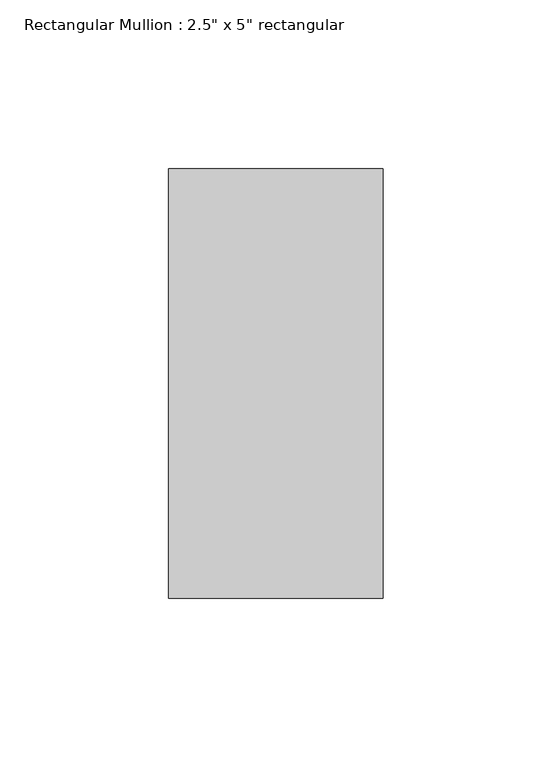
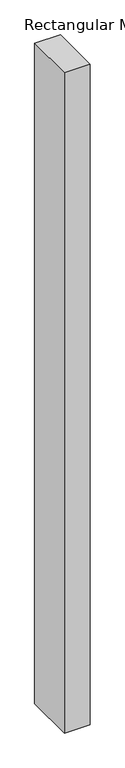
"""IFC4 building model written with IfcOpenShell, lengths in millimetres: member geometry."""

from ifc_helpers import new_model, si_unit, frame, origin, place, context, project, spatial, polyline, outline, extrude, source, transform, mapped, element, save


def member_ac3a6214(model_context):
    return source(origin(), model_context, "Body", "SweptSolid", [
        extrude(outline(polyline([(0.0, 63.5), (0.0, -63.5), (-63.5, -63.5), (-63.5, 63.5), (0.0, 63.5)])), frame((0.0, 0.0, -1720.9325096), z_axis=(0.0, 0.0, 1.0), x_axis=(1.0, 0.0, 0.0)), (0.0, 0.0, 1.0), 1720.9325096),
    ])


if __name__ == "__main__":
    model = new_model("IFC4")
    model_context = context("Model", 3, world=origin())
    ifc_project = project(units=[si_unit("LENGTHUNIT", "METRE", prefix="MILLI")], contexts=[model_context])
    site = spatial("IfcSite", under=ifc_project)
    building = spatial("IfcBuilding", under=site)
    placement = place(None, origin())
    member_shape = member_ac3a6214(model_context)
    element("IfcMember", 1, ObjectType="Rectangular Mullion : 2.5\" x 5\" rectangular", at=placement, inside=building, context=model_context, shape_type="MappedRepresentation", body=[
        mapped(member_shape, transform((0.0, 0.0, 0.0), x_axis=(1.0, 0.0, 0.0), y_axis=(0.0, 1.0, 0.0), z_axis=(0.0, 0.0, 1.0))),
    ])
    save(model, "model.ifc")

# Revit data of these elements
# Type "Rectangular Mullion : 2.5\" x 5\" rectangular"
#   built-in parameter 1007304 = 0.416667 (stored number, unit not read)
#   built-in parameter 1007301 = 0.104167 (stored number, unit not read)
#   built-in parameter 1007300 = 0.104167 (stored number, unit not read)
# Element 1 (IfcMember, "Rectangular Mullion : 2.5\" x 5\" rectangular")
#   Materials on its faces: "Aluminum"
# Materials
#   "Aluminum": class "Metal", colour RGB 247 247 247, transparency 0, Description = "Aluminum 6061", Cost = 0
